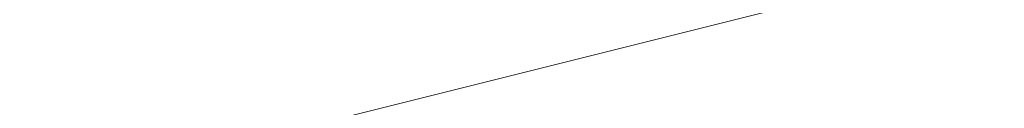
# Model space of a CAD drawing. Units: inches. Extents: x 2091 to 2899, y 967 to 2217.
# Tile 90 of 256: x 2251.2787 to 2251.31428, y 1099.92177 to 1099.9249. Entities that reach past the tile are written whole.
import ezdxf

# ---------------------------------------------------------------- set-up
doc = ezdxf.new("R2010")
doc.units = ezdxf.units.IN
doc.layers.add('A-ANNO-DIMS', color=2, linetype='Continuous', lineweight=18)
doc.layers.add('L-PLNT-TREE', color=94, linetype='Continuous', lineweight=13)
doc.layers.add('A-WALL-PATT', color=141, linetype='Continuous', lineweight=13, true_color=0xadddf7)
doc.styles.get("Standard").update_dxf_attribs({"font": 'arial.ttf'})
doc.dimstyles.new('ISO-25', dxfattribs={"dimtxt": 4, "dimasz": 4, "dimexe": 1.25, "dimexo": 0.625, "dimtad": 1, "dimdec": 0, "dimlunit": 3, "dimtxsty": 'Standard', "dimcen": 2.5, "dimadec": 0, "dimazin": 0, "dimtfac": 1, "dimtdec": 0, "dimtmove": 0, "dimatfit": 3, "dimfxl": 1, "dimarcsym": 0})

# ---------------------------------------------------------------- blocks, each defined once
blk = doc.blocks.new('*U29')
blk.add_line((-402.336, 12.192), (-451.104, 0))
blk = doc.blocks.new('*D71')
at = {"layer": 'A-ANNO-DIMS', "color": 0, "lineweight": -2, "transparency": 16777216}
for p, q in [((2212.143603, 1351.294059), (2212.143603, 969.464303)), ((2452.143603, 1351.294059), (2452.143603, 969.464303)), ((2216.143603, 970.714303), (2448.143603, 970.714303))]:
    blk.add_line(p, q, dxfattribs=at)
at = {"layer": 'A-ANNO-DIMS', "color": 0, "transparency": 16777216}
for points in [[(2216.143603, 971.38097), (2216.143603, 970.047636), (2212.143603, 970.714303)], [(2448.143603, 971.38097), (2448.143603, 970.047636), (2452.143603, 970.714303)]]:
    blk.add_solid(points, dxfattribs=at)
at = {"layer": 'Defpoints', "color": 0, "transparency": 16777216}
for p in [(2212.143603, 1351.919059), (2452.143603, 1351.919059), (2452.143603, 970.714303)]:
    blk.add_point(p, dxfattribs=at)
at = {"layer": 'A-ANNO-DIMS', "color": 0, "transparency": 16777216, "insert": (2332.143603, 973.381595), "char_height": 4, "attachment_point": 5}
blk.add_mtext('20\'-0"', dxfattribs=at)
blk = doc.blocks.new('*D75')
at = {"layer": 'A-ANNO-DIMS', "color": 0, "lineweight": -2, "transparency": 16777216}
for p, q in [((2212.143603, 1274.794059), (2212.143603, 969.464303)), ((2308.143603, 1274.794059), (2308.143603, 969.464303)), ((2216.143603, 970.714303), (2304.143603, 970.714303))]:
    blk.add_line(p, q, dxfattribs=at)
at = {"layer": 'A-ANNO-DIMS', "color": 0, "transparency": 16777216}
for points in [[(2216.143603, 971.38097), (2216.143603, 970.047636), (2212.143603, 970.714303)], [(2304.143603, 971.38097), (2304.143603, 970.047636), (2308.143603, 970.714303)]]:
    blk.add_solid(points, dxfattribs=at)
at = {"layer": 'Defpoints', "color": 0, "transparency": 16777216}
for p in [(2212.143603, 1275.419059), (2308.143603, 1275.419059), (2308.143603, 970.714303)]:
    blk.add_point(p, dxfattribs=at)
at = {"layer": 'A-ANNO-DIMS', "color": 0, "transparency": 16777216, "insert": (2260.143603, 973.381595), "char_height": 4, "attachment_point": 5}
blk.add_mtext('8\'-0"', dxfattribs=at)

msp = doc.modelspace()

# ---------------------------------------------------------------- hatches: boundary and pattern name
at = {"layer": 'A-WALL-PATT'}
h = msp.add_hatch(color=256, dxfattribs=at)
h.dxf.hatch_style = 1
h.paths.add_polyline_path([(2803.143603, 2050.919059), (2203.143603, 2050.919059), (2203.143603, 1090.919059), (2803.143603, 1090.919059)])
h.paths.add_polyline_path([(2635.79885, 1147.540465), (2674.524052, 1147.540465, 0.376086), (2678.529665, 1152.880202), (2678.529665, 1159.556473, 0.333335), (2674.524319, 1163.561846), (2674.524319, 1163.56185), (2674.524319, 1192.93439), (2635.805971, 1192.93439), (2597.087622, 1192.93439), (2597.087622, 1163.561846, 0.333335), (2593.082276, 1159.556473), (2593.082276, 1152.880202, 0.376086), (2597.087889, 1147.540465)], flags=0)
h.paths.add_polyline_path([(2436.010433, 1278.240778, 0.000483), (2435.952643, 1278.215027, -0.001328), (2435.935625, 1278.111693, -0.001711), (2436.11644, 1278.040758, 0.002185)], flags=0)
h.paths.add_polyline_path([(2794.143603, 1143.419059), (2794.143603, 1347.419059), (2543.370171, 1347.419059), (2543.370171, 1351.919059), (2794.143603, 1351.919059), (2794.143603, 1392.713555), (2793.947398, 1392.713555), (2793.947398, 1473.5369), (2794.143603, 1473.5369), (2794.143603, 1531.919059), (2650.143603, 1531.919059), (2650.143603, 1536.419059), (2794.143603, 1536.419059), (2794.143603, 1692.419059), (2609.375609, 1692.419059), (2609.375609, 1644.419059), (2604.875609, 1644.419059), (2604.875609, 1744.919059), (2609.375609, 1744.919059), (2609.375609, 1696.919059), (2794.143603, 1696.919059), (2794.143603, 1780.919059), (2609.643603, 1780.919059), (2493.875609, 1780.919059), (2493.875609, 1785.419059), (2609.643603, 1785.419059), (2794.143603, 1785.419059), (2794.143603, 1847.938821), (2793.951222, 1847.938821), (2793.951222, 1928.762166), (2794.143603, 1928.762166), (2794.143603, 1941.419059), (2614.143603, 1941.419059), (2614.143603, 1821.419059), (2609.643603, 1821.419059), (2609.643603, 1941.419059), (2392.143603, 1941.419059), (2392.143603, 1819.919059), (2387.643603, 1819.919059), (2387.643603, 1941.419059), (2212.143603, 1941.419059), (2212.143603, 1783.919059), (2392.143603, 1783.919059), (2392.143603, 1780.919059), (2212.143603, 1780.919059), (2212.143603, 1629.419059), (2387.643603, 1629.419059), (2387.643603, 1744.919059), (2392.143603, 1744.919059), (2392.143603, 1627.919059), (2317.143603, 1627.919059), (2317.143603, 1551.419059), (2317.143603, 1536.419059), (2459.383591, 1536.419059), (2459.383591, 1602.39648), (2463.883591, 1602.39648), (2463.883591, 1531.919059), (2456.643603, 1531.919059), (2456.643603, 1529.919059), (2452.143603, 1529.919059), (2452.143603, 1531.919059), (2312.643603, 1531.919059), (2312.643603, 1551.419059), (2306.143603, 1551.419059), (2306.143603, 1555.919059), (2308.143603, 1555.919059), (2308.143603, 1551.419059), (2312.643603, 1551.419059), (2312.643603, 1627.919059), (2212.143603, 1627.919059), (2212.143603, 1555.919059), (2270.143603, 1555.919059), (2270.143603, 1551.419059), (2212.143603, 1551.419059), (2212.143603, 1351.919059), (2272.143603, 1351.919059), (2272.143603, 1347.419059), (2212.143603, 1347.419059), (2212.143603, 1275.419059), (2308.143603, 1275.419059), (2308.143603, 1351.919059), (2452.143603, 1351.919059), (2452.143603, 1493.919059), (2456.643603, 1493.919059), (2456.643603, 1347.419059), (2312.643603, 1347.419059), (2312.643603, 1270.919059), (2212.143603, 1270.919059), (2212.143603, 1099.919059), (2281.237523, 1099.919059), (2282.871041, 1110.913803), (2282.008341, 1116.996603), (2278.557741, 1121.420403), (2268.205641, 1128.056203), (2272.087641, 1128.056203), (2273.812941, 1131.927003), (2279.420341, 1134.691903), (2285.027841, 1135.244903), (2287.615841, 1137.456803), (2288.047141, 1138.009803), (2289.341141, 1140.774703), (2291.066541, 1139.668703), (2292.360541, 1135.244903), (2295.379841, 1136.903803), (2296.242541, 1135.797903), (2297.105241, 1133.033003), (2300.124641, 1138.009803), (2303.143941, 1138.009803), (2304.437941, 1135.797903), (2303.143941, 1133.586003), (2306.594641, 1134.691903), (2307.888741, 1133.033003), (2310.908041, 1135.244903), (2313.927441, 1134.138903), (2315.62686, 1132.427102), (2308.320041, 1117.549603), (2290.203841, 1109.807903), (2288.909841, 1103.172103), (2289.272309, 1099.919059), (2434.918227, 1099.919059), (2431.593227, 1124.788059), (2429.930227, 1169.553059), (2430.927185, 1240.519694), (2435.658926, 1238.186126), (2437.135227, 1196.554059), (2438.798227, 1143.973059), (2442.678227, 1111.998059), (2446.558227, 1099.919059), (2794.143603, 1099.919059), (2794.143603, 1138.919059), (2548.032447, 1138.919059), (2548.032447, 1143.419059), (2548.032447, 1148.819059), (2546.668457, 1148.031559), (2528.685692, 1179.178622, 0.256256), (2512.032447, 1148.819059), (2512.032447, 1143.419059), (2512.032447, 1138.919059), (2507.532447, 1138.919059), (2507.532447, 1143.419059), (2507.532447, 1148.819059, 0.256256), (2490.879202, 1179.178622), (2472.896437, 1148.031559), (2471.532447, 1148.819059), (2471.532447, 1143.419059), (2467.032447, 1143.419059), (2467.032447, 1269.945786, 0.039061), (2460.909987, 1273.580059), (2467.032447, 1273.580059), (2467.032447, 1286.325364, 0.014511), (2465.216194, 1286.761905), (2467.032447, 1287.052576), (2467.032447, 1323.419059), (2471.532447, 1323.419059), (2471.532447, 1148.819059), (2489.532447, 1179.995973), (2490.896437, 1179.208473), (2490.879202, 1179.178622, -0.256256), (2507.532447, 1148.819059), (2507.532447, 1143.419059), (2512.032447, 1143.419059), (2512.032447, 1148.819059, -0.256256), (2528.685692, 1179.178622), (2528.668457, 1179.208473), (2530.032447, 1179.995973), (2548.032447, 1148.819059), (2548.032447, 1143.419059)], flags=16)
h.paths.add_polyline_path([(2607.768546, 1200.945083), (2607.768546, 1265.030625), (2597.087622, 1281.052011), (2619.784585, 1281.052011), (2627.795278, 1337.12686), (2635.79885, 1337.12686), (2643.816663, 1337.12686), (2651.827356, 1281.052011), (2674.524319, 1281.052011), (2663.843395, 1265.030625), (2663.843395, 1200.945083), (2635.805971, 1200.945083)], flags=0)
edge = h.paths.add_edge_path(flags=0)
edge.add_ellipse((13303.896215, 1272.998725), major_axis=(-10595.31304, 0.000001), ratio=0.842303870086, start_angle=0.6282372191, end_angle=0.6465540999, ccw=False)
edge.add_ellipse((2711.70045, 1156.852678), major_axis=(2.219769, 0), ratio=0.84230387, start_angle=111.535244, end_angle=180.628237, ccw=False)
edge.add_ellipse((13303.156292, 1272.998725), major_axis=(-10593.026306, 0), ratio=0.842303869544, start_angle=0.5282714718, end_angle=0.6465540971, ccw=False)
edge.add_line((2710.764596, 1175.333295), (2710.129986, 1175.333295))
edge.add_ellipse((2710.129986, 1176.579775), major_axis=(1.479846, 0), ratio=0.84230387, start_angle=180, end_angle=270, ccw=False)
edge.add_line((2708.65014, 1176.579775), (2708.65014, 1200.782914))
edge.add_ellipse((2710.129986, 1200.782914), major_axis=(1.479846, 0), ratio=0.84230387, start_angle=90, end_angle=180, ccw=False)
edge.add_line((2710.129986, 1202.029394), (2710.465075, 1202.029394))
edge.add_ellipse((13303.156292, 1272.998725), major_axis=(-10593.026306, 0), ratio=0.842303869544, start_angle=-0.0902290886, end_angle=0.3838667788, ccw=False)
edge.add_ellipse((2710.129986, 1290.927031), major_axis=(-1.479846, 0), ratio=0.84230387, start_angle=0, end_angle=90, ccw=False)
edge.add_line((2708.65014, 1290.927031), (2708.65014, 1315.13017))
edge.add_ellipse((2710.129986, 1315.13017), major_axis=(-1.479846, 0), ratio=0.84230387, start_angle=-90, end_angle=0, ccw=False)
edge.add_line((2710.129986, 1316.37665), (2710.706314, 1316.37665))
edge.add_ellipse((3238.40172, 1296.289566), major_axis=(528.234, 0), ratio=0.8423038695, start_angle=176.34957241, end_angle=177.82004969, ccw=False)
edge.add_ellipse((2775.063043, 1071.450696), major_axis=(313.307761, 0), ratio=0.8423038695, start_angle=102.12596555, end_angle=103.78052899, ccw=False)
edge.add_ellipse((2775.063043, 1078.305698), major_axis=(-305.302891, 0), ratio=0.8423038695, start_angle=-79.790461, end_angle=-77.55537271, ccw=False)
edge.add_ellipse((2695.141767, 1541.975383), major_axis=(-250.960216, 0), ratio=0.8423038695, start_angle=99.25656601, end_angle=102.55493264)
edge.add_line((2741.410326, 1334.214255), (2747.132545, 1337.378477))
edge.add_ellipse((2747.538616, 1336.857478), major_axis=(-0.739923, 0), ratio=0.8423039, start_angle=270, end_angle=307.93313, ccw=False)
edge.add_ellipse((2747.538616, 1336.857478), major_axis=(-0.739923, 0), ratio=0.8423039, start_angle=232.06687, end_angle=270, ccw=False)
edge.add_line((2747.944687, 1337.378477), (2753.666906, 1334.214255))
edge.add_ellipse((2799.935466, 1541.975383), major_axis=(250.960216, 0), ratio=0.8423038695, start_angle=257.44506736, end_angle=260.74343399)
edge.add_ellipse((2720.014189, 1078.305698), major_axis=(305.302891, 0), ratio=0.8423038695, start_angle=77.55537271, end_angle=79.790461, ccw=False)
edge.add_ellipse((2720.014189, 1071.450696), major_axis=(-313.307761, 0), ratio=0.8423038695, start_angle=256.21947101, end_angle=257.87403445, ccw=False)
edge.add_ellipse((2256.675512, 1296.289566), major_axis=(-528.234, 0), ratio=0.8423038695, start_angle=182.17995031, end_angle=183.65042759, ccw=False)
edge.add_line((2784.370918, 1316.37665), (2784.947247, 1316.37665))
edge.add_ellipse((2784.947247, 1315.13017), major_axis=(1.479846, 0), ratio=0.84230387, start_angle=0, end_angle=90, ccw=False)
edge.add_line((2786.427093, 1315.13017), (2786.427093, 1290.927031))
edge.add_ellipse((2784.947247, 1290.927031), major_axis=(1.479846, 0), ratio=0.84230387, start_angle=270, end_angle=360, ccw=False)
edge.add_ellipse((-7808.07906, 1272.998725), major_axis=(10593.026306, 0), ratio=0.842303869544, start_angle=-0.3838667788, end_angle=0.0902290886, ccw=False)
edge.add_line((2784.612157, 1202.029394), (2784.947247, 1202.029394))
edge.add_ellipse((2784.947247, 1200.782914), major_axis=(1.479846, 0), ratio=0.84230387, start_angle=0, end_angle=90, ccw=False)
edge.add_line((2786.427093, 1200.782914), (2786.427093, 1176.579775))
edge.add_ellipse((2784.947247, 1176.579775), major_axis=(-1.479846, 0), ratio=0.84230387, start_angle=90, end_angle=180, ccw=False)
edge.add_line((2784.947247, 1175.333295), (2784.312636, 1175.333295))
edge.add_ellipse((-7808.07906, 1272.998725), major_axis=(10593.026306, 0), ratio=0.842303869544, start_angle=-0.6186431963, end_angle=-0.5282714718, ccw=False)
edge.add_ellipse((2783.376783, 1156.852678), major_axis=(-2.219769, 0), ratio=0.84230387, start_angle=179.371763, end_angle=248.464757, ccw=False)
edge.add_ellipse((-7808.818983, 1272.998725), major_axis=(-10595.31304, 0.000004), ratio=0.842303865762, start_angle=179.3534459226, end_angle=179.3717628034, ccw=False)
edge.add_ellipse((2780.297303, 1153.500793), major_axis=(-5.246426, 0), ratio=0.84230387, start_angle=90, end_angle=179.353446, ccw=False)
edge.add_line((2780.297303, 1149.081708), (2714.77993, 1149.081708))
edge.add_ellipse((2714.77993, 1153.500793), major_axis=(5.246426, 0), ratio=0.84230387, start_angle=180.646554, end_angle=270, ccw=False)
edge = h.paths.add_edge_path(flags=0)
edge.add_line((2718.187367, 1151.007833), (2718.187367, 1170.472364))
edge.add_ellipse((2721.14706, 1170.472364), major_axis=(-2.959692, 0), ratio=0.84230387, start_angle=-90, end_angle=0, ccw=False)
edge.add_line((2721.14706, 1172.965324), (2773.930173, 1172.965324))
edge.add_ellipse((2773.930173, 1170.472364), major_axis=(-2.959692, 0), ratio=0.84230387, start_angle=180, end_angle=270, ccw=False)
edge.add_line((2776.889865, 1170.472364), (2776.889865, 1151.007833))
edge.add_line((2776.889865, 1151.007833), (2718.187367, 1151.007833))
edge = h.paths.add_edge_path(flags=0)
edge.add_line((2718.187367, 1180.23415), (2718.187367, 1199.057834))
edge.add_ellipse((2747.538616, 1320.39864), major_axis=(147.017924, 0), ratio=0.8423038695, start_angle=256.40186531, end_angle=283.59813469)
edge.add_line((2776.889865, 1199.057834), (2776.889865, 1180.23415))
edge.add_ellipse((2747.538616, 1301.574956), major_axis=(147.017924, 0), ratio=0.8423038695, start_angle=256.40186531, end_angle=283.59813469, ccw=False)
edge = h.paths.add_edge_path(flags=0)
edge.add_ellipse((13303.156292, 1272.998725), major_axis=(-10591.54646, 0), ratio=0.842303869555, start_angle=0.0555943135, end_angle=0.3777641939, ccw=False)
edge.add_line((2711.616859, 1262.72171), (2715.667408, 1249.495396))
edge.add_ellipse((6413.891963, 1241.691919), major_axis=(-3698.236159, 0), ratio=0.84230386955, start_angle=-0.120897369, end_angle=0.364076349)
edge.add_line((2715.761038, 1218.192455), (2711.934307, 1203.167361))
edge = h.paths.add_edge_path(flags=0)
edge.add_line((2718.187367, 1251.074566), (2716.002485, 1267.450435))
edge.add_ellipse((2742.151175, 1202.18954), major_axis=(81.772585, 0), ratio=0.84230387, start_angle=94.27742096, end_angle=111.8349538, ccw=False)
edge.add_line((2737.009748, 1270.930626), (2758.067484, 1270.930626))
edge.add_ellipse((2752.926058, 1202.18954), major_axis=(81.772585, 0), ratio=0.84230387, start_angle=68.1650462, end_angle=85.72257904, ccw=False)
edge.add_line((2779.074747, 1267.450435), (2776.889865, 1251.074566))
edge.add_ellipse((2750.338059, 1187.885356), major_axis=(79.579664, 0), ratio=0.84230387, start_angle=67.20808512, end_angle=85.1299304)
edge.add_line((2756.034656, 1254.743656), (2739.042576, 1254.743656))
edge.add_ellipse((2744.739174, 1187.885356), major_axis=(79.579664, 0), ratio=0.84230387, start_angle=94.8700696, end_angle=112.79191488)
edge = h.paths.add_edge_path(flags=0)
edge.add_line((2783.142926, 1203.167361), (2779.316194, 1218.192455))
edge.add_ellipse((-918.81473, 1241.691919), major_axis=(3698.236159, 0), ratio=0.84230386955, start_angle=-0.364076349, end_angle=0.120897369)
edge.add_line((2779.409825, 1249.495396), (2783.460373, 1262.72171))
edge.add_ellipse((-7808.07906, 1272.998725), major_axis=(-10591.54646, 0), ratio=0.84230386954, start_angle=179.6222358061, end_angle=179.9444056865, ccw=False)
edge = h.paths.add_edge_path(flags=0)
edge.add_ellipse((2734.200892, 1286.69044), major_axis=(-0.356609, 6.340078), ratio=0.60383358, start_angle=89.0020143, end_angle=253.657408, ccw=False)
edge.add_line((2730.369001, 1286.541806), (2730.369001, 1301.35198))
edge.add_line((2730.369001, 1301.35198), (2735.913311, 1305.214803))
edge.add_ellipse((2736.384917, 1304.734561), major_axis=(0.739923, 0), ratio=0.8423039, start_angle=90, end_angle=134.480211, ccw=False)
edge.add_line((2736.384917, 1305.357801), (2738.032783, 1305.357801))
edge.add_line((2738.032783, 1305.357801), (2738.032783, 1307.707927))
edge.add_ellipse((2794.201642, 1307.707927), major_axis=(56.168859, 0), ratio=0.84230387, start_angle=150.5614304, end_angle=180, ccw=False)
edge.add_ellipse((2700.875591, 1307.707927), major_axis=(-56.168859, 0), ratio=0.84230387, start_angle=180, end_angle=209.4385696, ccw=False)
edge.add_line((2757.04445, 1307.707927), (2757.04445, 1305.357801))
edge.add_line((2757.04445, 1305.357801), (2758.692316, 1305.357801))
edge.add_ellipse((2758.692316, 1304.734561), major_axis=(-0.739923, 0), ratio=0.8423039, start_angle=225.519789, end_angle=270, ccw=False)
edge.add_line((2759.163922, 1305.214803), (2764.708231, 1301.35198))
edge.add_line((2764.708231, 1301.35198), (2764.708231, 1286.541806))
edge.add_ellipse((2760.87634, 1286.69044), major_axis=(0.356609, 6.340078), ratio=0.60383358, start_angle=106.342592, end_angle=270.9979857, ccw=False)
edge.add_line((2757.04445, 1285.79709), (2757.04445, 1307.707927))
edge.add_ellipse((2700.875591, 1307.707927), major_axis=(-56.168859, 0), ratio=0.84230387, start_angle=180, end_angle=209.4385696)
edge.add_ellipse((2794.201642, 1307.707927), major_axis=(56.168859, 0), ratio=0.84230387, start_angle=150.5614304, end_angle=180)
edge.add_line((2738.032783, 1307.707927), (2738.032783, 1285.79709))
h.paths.add_polyline_path([(2417.812273, 1104.449704), (2413.492273, 1102.529704), (2410.612273, 1103.969704), (2409.172273, 1106.369704), (2407.252273, 1107.329704), (2406.292273, 1109.729704), (2405.332273, 1114.049704), (2405.332273, 1117.889704), (2406.292273, 1120.129704), (2407.252273, 1119.809704), (2408.848322, 1118.327658), (2410.173945, 1119.42417), (2410.211273, 1120.405704), (2411.040731, 1121.419054), (2410.699273, 1119.858704), (2410.173945, 1119.42417), (2410.088452, 1117.176109), (2411.132836, 1116.206324), (2413.972273, 1119.329704), (2416.852273, 1120.769704), (2416.869721, 1120.798784), (2417.035071, 1119.405116), (2417.896213, 1118.143384), (2418.292273, 1118.369704), (2419.544447, 1120.039269), (2419.360915, 1118.387487), (2419.032108, 1119.356151), (2418.398939, 1118.511926), (2419.252273, 1114.529704), (2418.794091, 1107.198795)], flags=0)
h.paths.add_polyline_path([(2508.870171, 1347.419059), (2508.370171, 1347.419059), (2508.370171, 1351.919059), (2508.870171, 1351.919059)], flags=0)
h.paths.add_polyline_path([(2473.370171, 1347.419059), (2472.370171, 1347.419059), (2467.870171, 1347.419059), (2467.870171, 1455.419059), (2472.370171, 1455.419059), (2472.370171, 1352.419059), (2473.370171, 1352.419059)], flags=0)
h.paths.add_polyline_path([(2352.106244, 1217.446197), (2349.226244, 1218.886197), (2347.786244, 1221.286197), (2345.866244, 1222.246197), (2344.906244, 1224.646197), (2343.946244, 1228.966197), (2343.946244, 1232.806197), (2344.906244, 1235.046197), (2345.866244, 1234.726197), (2347.462293, 1233.244152), (2348.787916, 1234.340663), (2348.825244, 1235.322197), (2349.654702, 1236.335547), (2349.313244, 1234.775197), (2348.787916, 1234.340663), (2348.702423, 1232.092603), (2349.746807, 1231.122817), (2352.586244, 1234.246197), (2355.466244, 1235.686197), (2355.483692, 1235.715277), (2355.649043, 1234.321609), (2356.510185, 1233.059877), (2356.906244, 1233.286197), (2358.158418, 1234.955762), (2357.974887, 1233.30398), (2357.646079, 1234.272644), (2357.012911, 1233.428419), (2357.866244, 1229.446197), (2357.408062, 1222.115288), (2356.426244, 1219.366197)], flags=0)
h.paths.add_polyline_path([(2348.2968, 1112.22442), (2347.0138, 1112.31042), (2345.5298, 1114.12742), (2345.7318, 1115.85842), (2346.8118, 1116.98242), (2346.8118, 1114.64642), (2345.8668, 1114.21442), (2346.8798, 1114.30042)], flags=0)
h.paths.add_polyline_path([(2347.0138, 1110.92642), (2346.2718, 1110.49342), (2346.6098, 1111.18642)], flags=0)
h.paths.add_polyline_path([(2345.8668, 1118.19442), (2345.5298, 1117.32942), (2343.7078, 1118.02142), (2344.3828, 1118.62642)], flags=0)
h.paths.add_polyline_path([(2346.6768, 1109.28242), (2346.0698, 1108.07142), (2345.8668, 1110.06142)], flags=0)
h.paths.add_polyline_path([(2345.0568, 1119.75142), (2343.6398, 1119.75142), (2343.9778, 1121.13542)], flags=0)
h.paths.add_polyline_path([(2345.2598, 1116.55042), (2345.1248, 1115.85842), (2344.9218, 1115.68542), (2344.7198, 1116.37742)], flags=0)
h.paths.add_polyline_path([(2345.6648, 1112.31042), (2345.4618, 1111.53242), (2344.0448, 1111.96442), (2344.6518, 1112.57042)], flags=0)
h.paths.add_polyline_path([(2345.1918, 1113.34942), (2344.4498, 1113.86842), (2344.7198, 1114.38742)], flags=0)
h.paths.add_polyline_path([(2344.6518, 1116.80942), (2344.1798, 1115.68542), (2344.6518, 1115.33942), (2343.9098, 1114.90642), (2343.0328, 1115.94442), (2343.6398, 1116.46342)], flags=0)
h.paths.add_polyline_path([(2345.8668, 1106.68642), (2344.9898, 1105.56242), (2344.5168, 1106.60042)], flags=0)
h.paths.add_polyline_path([(2344.8548, 1110.06142), (2344.5168, 1109.28242), (2344.1128, 1109.71542)], flags=0)
h.paths.add_polyline_path([(2344.0448, 1113.52242), (2343.4378, 1113.08942), (2342.7628, 1113.95442)], flags=0)
h.paths.add_polyline_path([(2344.3148, 1111.01242), (2342.9648, 1110.32042), (2342.9648, 1111.09942)], flags=0)
h.paths.add_polyline_path([(2345.1248, 1104.69742), (2344.5848, 1103.74542), (2344.4498, 1104.26442)], flags=0)
h.paths.add_polyline_path([(2342.8298, 1121.22242), (2341.7498, 1120.53042), (2340.5358, 1121.04942), (2340.1308, 1121.82842), (2340.6708, 1122.95242), (2341.1428, 1121.82842), (2341.6148, 1122.00142)], flags=0)
h.paths.add_polyline_path([(2342.9648, 1119.75142), (2343.0328, 1118.45342), (2342.0878, 1118.02142), (2342.0198, 1119.49142)], flags=0)
h.paths.add_polyline_path([(2342.6948, 1116.89642), (2341.9528, 1116.63642), (2342.0198, 1117.32942)], flags=0)
h.paths.add_polyline_path([(2343.0328, 1112.22442), (2342.0198, 1111.79142), (2341.5478, 1112.22442), (2342.3578, 1113.34942)], flags=0)
h.paths.add_polyline_path([(2343.7748, 1104.43742), (2342.6278, 1102.88042), (2342.6948, 1104.61042), (2343.4378, 1105.12942)], flags=0)
h.paths.add_polyline_path([(2342.0198, 1115.07942), (2340.8058, 1115.51242), (2340.9408, 1116.37742)], flags=0)
h.paths.add_polyline_path([(2341.4808, 1120.09742), (2341.4808, 1119.40542), (2341.0758, 1119.57842), (2341.1428, 1120.09742)], flags=0)
h.paths.add_polyline_path([(2341.8178, 1114.47342), (2340.9408, 1113.08942), (2340.8058, 1114.56042)], flags=0)
h.paths.add_polyline_path([(2341.1428, 1118.54042), (2340.9408, 1116.98242), (2339.0508, 1117.67542), (2339.0508, 1118.62642)], flags=0)
h.paths.add_polyline_path([(2342.6948, 1101.66842), (2341.9528, 1101.84142), (2342.5598, 1102.36142)], flags=0)
h.paths.add_polyline_path([(2340.3328, 1119.66542), (2338.4438, 1119.57842), (2337.9038, 1120.35742), (2339.6578, 1120.61642)], flags=0)
h.paths.add_polyline_path([(2340.3328, 1115.33942), (2340.0628, 1113.69542), (2339.3878, 1115.33942)], flags=0)
h.paths.add_polyline_path([(2341.8178, 1103.83142), (2341.5478, 1102.88042), (2341.1428, 1103.65842)], flags=0)
h.paths.add_polyline_path([(2339.0508, 1122.86642), (2337.2958, 1121.82842), (2337.0938, 1123.12542), (2337.7688, 1123.81842)], flags=0)
h.paths.add_polyline_path([(2339.1178, 1121.74142), (2338.8478, 1121.22242), (2338.1738, 1121.04942), (2338.3758, 1121.56842)], flags=0)
h.paths.add_polyline_path([(2339.1858, 1119.31942), (2338.6458, 1118.71342), (2338.2408, 1118.10742), (2338.2408, 1118.88642)], flags=0)
h.paths.add_polyline_path([(2341.1428, 1101.92842), (2340.6028, 1101.23642), (2340.0628, 1101.84142), (2340.6028, 1102.36142)], flags=0)
h.paths.add_polyline_path([(2337.6338, 1117.76142), (2336.6208, 1118.28042), (2337.2958, 1118.97242)], flags=0)
h.paths.add_polyline_path([(2336.8238, 1119.57842), (2334.7988, 1118.97242), (2335.2038, 1120.35742), (2336.5538, 1120.87642)], flags=0)
h.paths.add_polyline_path([(2339.1178, 1100.45742), (2337.3638, 1100.54342), (2336.7558, 1101.23642)], flags=0)
h.paths.add_polyline_path([(2336.3508, 1122.43342), (2336.0138, 1121.91442), (2334.9338, 1122.43342), (2334.5288, 1123.47142), (2335.7438, 1122.77942)], flags=0)
h.paths.add_polyline_path([(2334.7318, 1120.87642), (2334.2588, 1120.35742), (2334.0568, 1120.78942), (2334.5968, 1121.30842)], flags=0)
h.paths.add_polyline_path([(2334.4618, 1122.17442), (2332.5718, 1121.30842), (2331.3568, 1122.17442), (2332.0998, 1122.86642)], flags=0)
h.paths.add_polyline_path([(2334.2588, 1118.54042), (2333.3818, 1118.45342), (2333.6518, 1119.31942)], flags=0)
h.paths.add_polyline_path([(2335.5418, 1102.27442), (2334.1918, 1102.62042), (2335.2718, 1103.31242)], flags=0)
h.paths.add_polyline_path([(2332.7068, 1119.66542), (2331.6948, 1120.44342), (2332.5048, 1120.78942)], flags=0)
h.paths.add_polyline_path([(2334.7318, 1101.14942), (2333.5168, 1101.58242), (2333.9888, 1101.75542)], flags=0)
h.paths.add_polyline_path([(2332.6398, 1116.63642), (2331.0868, 1116.29042), (2331.9648, 1118.19442)], flags=0)
h.paths.add_polyline_path([(2330.7498, 1121.56842), (2330.2768, 1120.27042), (2328.5228, 1119.31942), (2328.9948, 1121.04942)], flags=0)
h.paths.add_polyline_path([(2330.7498, 1118.62642), (2330.0078, 1117.50242), (2329.8728, 1118.02142)], flags=0)
h.paths.add_polyline_path([(2332.0998, 1102.36142), (2330.5468, 1102.01442), (2331.6948, 1102.96642)], flags=0)
h.paths.add_polyline_path([(2329.5348, 1113.60842), (2329.0628, 1112.31042), (2328.5898, 1113.34942)], flags=0)
h.paths.add_polyline_path([(2328.3878, 1117.84842), (2327.5098, 1116.55042), (2327.1728, 1117.76142)], flags=0)
h.paths.add_polyline_path([(2329.7378, 1106.51342), (2329.5348, 1105.30242), (2328.2528, 1106.08142)], flags=0)
h.paths.add_polyline_path([(2328.6578, 1114.38742), (2328.0498, 1114.12742), (2328.3198, 1114.90642)], flags=0)
h.paths.add_polyline_path([(2328.3198, 1112.22442), (2327.1058, 1112.13742), (2326.7008, 1112.65642)], flags=0)
h.paths.add_polyline_path([(2326.9028, 1115.25242), (2326.7008, 1114.12742), (2325.2158, 1113.60842), (2326.0928, 1115.33942)], flags=0)
h.paths.add_polyline_path([(2326.6328, 1108.33042), (2326.0928, 1107.37942), (2325.8908, 1108.50342), (2326.4978, 1109.10942)], flags=0)
h.paths.add_polyline_path([(2615.143603, 1531.919059), (2609.643603, 1531.919059), (2609.643603, 1620.419059), (2614.143603, 1620.419059), (2614.143603, 1536.419059), (2615.143603, 1536.419059)], flags=0)
h.paths.add_polyline_path([(2545.143603, 1563.419059), (2464.143603, 1563.419059), (2464.143603, 1632.419059), (2509.143603, 1632.419059), (2509.143603, 1627.919059), (2509.143603, 1603.919059), (2468.643603, 1603.919059), (2468.643603, 1567.919059), (2540.643603, 1567.919059), (2540.643603, 1591.919059), (2545.143603, 1591.919059)], flags=0)
h.paths.add_polyline_path([(2388.969048, 1549.985735), (2357.434181, 1549.985735), (2357.434181, 1623.360778), (2399.362777, 1623.360778), (2435.689465, 1623.360778), (2435.592547, 1602.559273), (2435.592547, 1602.39648), (2388.969048, 1602.39648)], flags=0)
h.paths.add_polyline_path([(2388.880628, 1555.809151), (2374.904429, 1555.809151), (2374.904429, 1600.571564), (2374.904429, 1615.457645), (2406.350877, 1615.457645), (2406.350877, 1618.939431), (2412.174293, 1615.457645), (2406.350877, 1611.97586), (2406.350877, 1615.457645), (2388.880628, 1615.457645)], flags=0)
h.paths.add_polyline_path([(2568.875609, 1644.419059), (2453.375609, 1644.419059), (2453.375609, 1785.419059), (2457.875609, 1785.419059), (2457.875609, 1648.919059), (2568.875609, 1648.919059)], flags=0)
h.paths.add_polyline_path([(2212.143603, 1945.919059), (2212.143603, 2041.919059), (2794.143603, 2041.919059), (2794.143603, 1945.919059)], flags=16)
h.paths.add_polyline_path([(2271.082728, 1964.317238), (2776.852968, 1964.317238), (2776.852968, 2037.169623), (2271.082728, 2037.169623)], flags=8)
h.paths.add_polyline_path([(2380.649285, 1536.824144), (2461.040809, 1536.824144), (2461.040809, 1554.652587), (2380.649285, 1554.652587)], flags=8)
h.paths.add_polyline_path([(2240.755709, 1609.725451), (2309.185829, 1609.725451), (2309.185829, 1617.698204), (2240.755709, 1617.698204)], flags=8)
h.paths.add_polyline_path([(2212.677255, 1313.504102), (2282.59152, 1313.504102), (2282.59152, 1322.745239), (2212.677255, 1322.745239)], flags=8)
h.paths.add_polyline_path([(2457.111976, 1114.778574), (2558.481581, 1114.778574), (2558.481581, 1142.219682), (2457.111976, 1142.219682)], flags=8)
h.paths.add_polyline_path([(2473.442337, 1273.010067), (2604.641226, 1273.010067), (2604.641226, 1318.346935), (2473.442337, 1318.346935)], flags=8)
h.paths.add_polyline_path([(2638.876302, 1626.977432), (2684.250367, 1627.976738), (2684.038483, 1637.597494), (2638.664417, 1636.598188)], flags=8)
h.paths.add_polyline_path([(2537.590554, 1453.793447), (2628.389547, 1453.793447), (2628.389547, 1475.344811), (2537.590554, 1475.344811)], flags=8)
h.paths.add_polyline_path([(2504.137638, 1714.632397), (2554.647187, 1714.632397), (2554.647187, 1730.237712), (2504.137638, 1730.237712)], flags=8)
h.paths.add_polyline_path([(2487.501181, 1575.651872), (2535.097121, 1575.651872), (2535.097121, 1598.377646), (2487.501181, 1598.377646)], flags=8)
h.paths.add_polyline_path([(2709.0994, 1735.710278), (2740.016601, 1735.710278), (2740.016601, 1749.937641), (2709.0994, 1749.937641)], flags=8)
h.paths.add_polyline_path([(2442.438424, 1792.171657), (2564.728835, 1792.171657), (2564.728835, 1842.000163), (2442.438424, 1842.000163)], flags=8)
h.paths.add_polyline_path([(2655.815801, 1809.644076), (2789.520142, 1806.693796), (2790.084977, 1832.291638), (2656.380635, 1835.241918)], flags=8)
h.paths.add_polyline_path([(2234.842697, 1797.720143), (2368.592851, 1794.768852), (2369.160718, 1820.504132), (2235.410564, 1823.455423)], flags=8)
h.paths.add_polyline_path([(2245.138466, 1644.006335), (2398.427733, 1640.6239), (2398.994842, 1666.32482), (2245.705575, 1669.707255)], flags=8)
h.paths.add_polyline_path([(2306.142847, 1431.168519), (2413.768314, 1428.793687), (2414.333148, 1454.391529), (2306.707682, 1456.76636)], flags=8)
h.paths.add_polyline_path([(2306.834582, 1458.233145), (2393.380484, 1456.323449), (2393.932808, 1481.354358), (2307.386907, 1483.264054)], flags=8)

# ---------------------------------------------------------------- block references
at = {"layer": 'L-PLNT-TREE', "xscale": 0.0393700787401575, "yscale": 0.0393700787401575, "zscale": 0.0393700787401575}
msp.add_blockref('*U29', (2269.041014, 1099.919059), dxfattribs=at)

# ---------------------------------------------------------------- dimensions: what is measured, and where the dimension line sits
at = {"layer": 'A-ANNO-DIMS'}
for base, p1, p2, picture, middle in [((2452.143603, 970.714303), (2212.143603, 1351.919059), (2452.143603, 1351.919059), '*D71', (2332.143603, 973.381595)), ((2308.143603, 970.714303), (2212.143603, 1275.419059), (2308.143603, 1275.419059), '*D75', (2260.143603, 973.381595))]:
    dim = msp.add_linear_dim(base=base, p1=p1, p2=p2, dimstyle='ISO-25', override={"dimdec": 1, "dimlfac": 1, "dimrnd": 0, "dimzin": 1, "dimdsep": 46, "dimlunit": 4, "dimfrac": 2}, dxfattribs=at)
    dim.commit()
    dim.dimension.update_dxf_attribs({"geometry": picture, "text_midpoint": middle})

doc.saveas('drawing.dxf')
